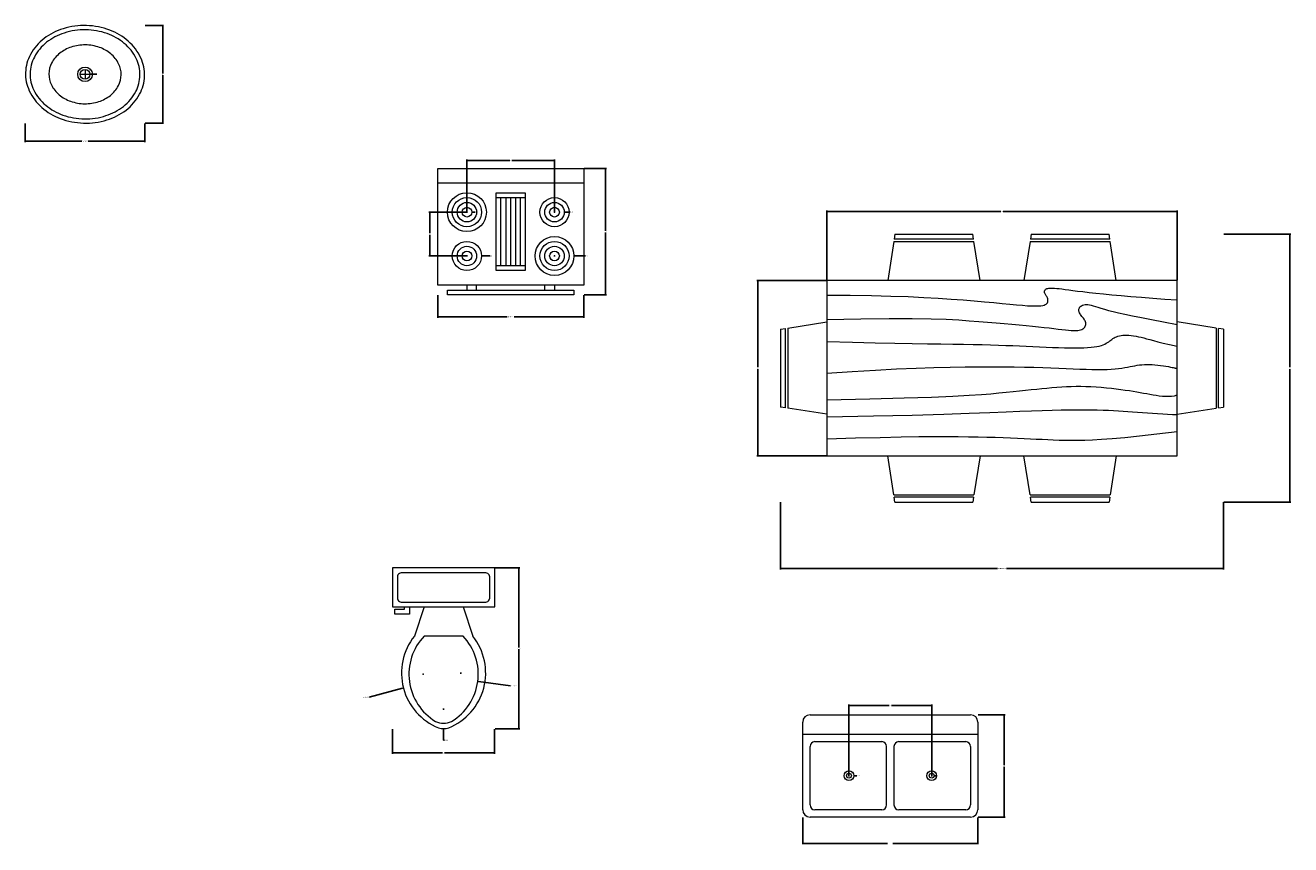
# Model space of a CAD drawing. Units: inches. Extents: x -52 to 1967, y 32 to 824.
# Tile 8 of 10: x 1561 to 1821, y 303 to 471. Entities that reach past the tile are written whole.
import ezdxf

# ---------------------------------------------------------------- set-up
doc = ezdxf.new("R2010")
doc.units = ezdxf.units.IN
for name, color, linetype, lineweight in [('A-ANNO-DIMS', 2, 'Continuous', 18), ('A-EQPM', 9, 'Continuous', 18), ('A-FLOR-FIXT', 9, 'Continuous', 18), ('A-FURN', 8, 'Continuous', 18)]:
    doc.layers.add(name, color=color, linetype=linetype, lineweight=lineweight)
doc.styles.get("Standard").update_dxf_attribs({"font": 'arial.ttf'})
doc.dimstyles.get("Standard").update_dxf_attribs({"dimtxt": 0.18, "dimasz": 0.18, "dimexe": 0.18, "dimexo": 0.0625, "dimgap": 0.09, "dimtad": 0, "dimtih": 1, "dimtoh": 1, "dimdec": 4, "dimzin": 0, "dimdsep": 46, "dimtxsty": 'Standard', "dimcen": 0.09, "dimadec": 0, "dimazin": 0, "dimtfac": 1, "dimtdec": 4, "dimtofl": 0, "dimtmove": 0, "dimatfit": 3, "dimfxl": 1, "dimtolj": 1, "dimtzin": 0, "dimarcsym": 0})

# ---------------------------------------------------------------- blocks, each defined once
blk = doc.blocks.new('Sink-double - 36 in top')
for p, q in [((-18, -4), (18, -4)), ((-0.75, -18.5), (-0.75, -6.5)), ((0.75, -6.5), (0.75, -18.5))]:
    blk.add_line(p, q)
for points in [[(-16.5, 0), (16.5, 0)], [(-18, -19.5), (-18, -1.5)], [(18, -1.5), (18, -19.5)], [(-16.5, -18.5), (-16.5, -6.5)], [(-15.5, -5.5), (-1.75, -5.5)], [(1.75, -5.5), (15.5, -5.5)], [(16.5, -6.5), (16.5, -18.5)], [(-1.75, -19.5), (-15.5, -19.5)], [(15.5, -19.5), (1.75, -19.5)], [(16.5, -21), (-16.5, -21)]]:
    blk.add_lwpolyline(points)
for centre, radius in [((-8.5, -12.5), 1), ((-8.5, -12.5), 0.5), ((8.5, -12.5), 1), ((8.5, -12.5), 0.5)]:
    blk.add_circle(centre, radius)
for centre, radius, start, end in [((-16.5, -1.5), 1.5, 90, 180), ((16.5, -1.5), 1.5, 0, 90), ((-15.5, -6.5), 1, 90, 180), ((-1.75, -6.5), 1, 0, 90), ((1.75, -6.5), 1, 90, 180), ((15.5, -6.5), 1, 0, 90), ((-16.5, -19.5), 1.5, 180, 270), ((-15.5, -18.5), 1, 180, 270), ((-1.75, -18.5), 1, 270, 0), ((1.75, -18.5), 1, 180, 270), ((15.5, -18.5), 1, 270, 0), ((16.5, -19.5), 1.5, 270, 0)]:
    blk.add_arc(centre, radius, start, end)
blk = doc.blocks.new('Range-Oven - 30 in top')
for p, q in [((0, -3), (30, -3)), ((12, -6), (18, -6)), ((13, -20), (13, -6)), ((14, -6), (14, -20)), ((15, -20), (15, -6)), ((16, -6), (16, -20)), ((17, -20), (17, -6)), ((18, -20), (12, -20)), ((6, -24), (6, -25)), ((8, -25), (8, -24)), ((22, -25), (22, -24)), ((24, -24), (24, -25))]:
    blk.add_line(p, q)
for points in [[(0, -24), (0, 0), (30, 0), (30, -24)], [(12, -21), (12, -5), (18, -5), (18, -21)], [(2, -26), (2, -25), (28, -25), (28, -26)]]:
    blk.add_lwpolyline(points, close=True)
for centre, radius in [((6, -9), 4), ((6, -9), 3), ((6, -9), 2), ((24, -9), 3), ((24, -9), 2), ((6, -9), 1), ((24, -9), 1), ((6, -18), 3), ((24, -18), 4), ((24, -18), 3), ((6, -18), 2), ((6, -18), 1), ((24, -18), 2), ((24, -18), 1)]:
    blk.add_circle(centre, radius)
blk = doc.blocks.new('Toilet - top')
for p, q in [((9.5, -6), (9.5, -2)), ((-10, -8.5), (-8, -8.5)), ((-10, -9.5), (-10, -8.5)), ((-7, -9.5), (-10, -9.5)), ((-8, -8.5), (-8, -8)), ((-7, -8), (-7, -9.5)), ((-4, -8), (-6, -14)), ((4, -8), (6, -14)), ((4, -14), (-4, -14))]:
    blk.add_line(p, q)
blk.add_lwpolyline([(10.5, -8), (10.5, 0), (-10.5, 0), (-10.5, -8)], close=True)
for points in [[(-9.5, -2), (-9.5, -6)], [(8.5, -1), (-8.5, -1)], [(-8.5, -7), (8.5, -7)]]:
    blk.add_lwpolyline(points)
for centre, radius, start, end in [((-8.62, -1.88), 0.884, 81.8699, 188.1301), ((8.62, -1.88), 0.884, 351.8699, 98.1301), ((-8.62, -6.12), 0.884, 171.8699, 278.1301), ((8.62, -6.12), 0.884, 261.8699, 8.1301), ((3.52, -21.58), 12.17, 141.4691, 247.9714), ((4.2, -21.82), 11.33, 136.3677, 238.9468), ((-3.52, -21.58), 12.17, 292.0284, 38.5307), ((-4.2, -21.82), 11.33, 301.053, 43.6321), ((0, -27.88), 4, 245.7318, 294.2682), ((0, -29), 4, 254.8605, 285.1395)]:
    blk.add_arc(centre, radius, start, end)
blk = doc.blocks.new('Sink - Oval top')
for p, q in [((-1, 0), (1, 0)), ((0, 1), (0, -1))]:
    blk.add_line(p, q)
for points in [[(-12.23, 0.39, 0.117634), (-11.46, -3.36, 0.104469), (-8.88, -6.8, 0.090016), (-5.08, -9.07, 0.08192), (-0.32, -10.02, 0.08192), (4.49, -9.38, 0.090016), (8.42, -7.36, 0.104469), (11.22, -4.09, 0.117634), (12.23, -0.39, 0.117634), (11.46, 3.36, 0.104469), (8.88, 6.8, 0.090016), (5.08, 9.07, 0.08192), (0.32, 10.02, 0.08192), (-4.49, 9.38, 0.090016), (-8.42, 7.36, 0.104469), (-11.22, 4.09, 0.117634)], [(-11.29, 0.16, 0.118622), (-10.52, -3.25, 0.104678), (-8.07, -6.36, 0.089562), (-4.54, -8.37, 0.081185), (-0.13, -9.15, 0.081185), (4.3, -8.49, 0.089562), (7.89, -6.58, 0.104678), (10.42, -3.55, 0.118622), (11.29, -0.16, 0.118622), (10.52, 3.25, 0.104678), (8.07, 6.36, 0.089562), (4.54, 8.37, 0.081185), (0.13, 9.15, 0.081185), (-4.3, 8.49, 0.089562), (-7.89, 6.58, 0.104678), (-10.42, 3.55, 0.118622)], [(-7.42, 0.08, 0.118283), (-6.91, -2.17, 0.104607), (-5.29, -4.21, 0.089718), (-2.97, -5.53, 0.081436), (-0.07, -6.04, 0.081436), (2.84, -5.59, 0.089718), (5.2, -4.33, 0.104607), (6.86, -2.32, 0.118283), (7.42, -0.08, 0.118283), (6.91, 2.17, 0.104607), (5.29, 4.21, 0.089718), (2.97, 5.53, 0.081436), (0.07, 6.04, 0.081436), (-2.84, 5.59, 0.089718), (-5.2, 4.33, 0.104607), (-6.86, 2.32, 0.118283)]]:
    blk.add_lwpolyline(points, format="xyb", close=True)
for radius in [1.5, 1]:
    blk.add_circle((0, 0), radius)
blk = doc.blocks.new('Dining Set - 36 x 72 in.')
for p, q in [((-22, 27.5), (-22.1562, 26.50042)), ((-5.8416, 26.5), (-22.1534, 26.5)), ((-22, 27.5), (-6, 27.5)), ((-5.8437, 26.49966), (-6, 27.5)), ((6, 27.5), (5.8438, 26.50042)), ((22.1584, 26.5), (5.8466, 26.5)), ((6, 27.5), (22, 27.5)), ((22.1563, 26.49966), (22, 27.5)), ((-22.2343, 26.00059), (-23.4847, 17.99762)), ((-22.2304, 26), (-5.7608, 26)), ((-4.5152, 17.99762), (-5.7655, 25.99926)), ((5.7657, 26.00059), (4.5153, 17.99762)), ((5.7696, 26), (22.2392, 26)), ((23.4848, 17.99762), (22.2345, 25.99926)), ((36, 18), (-36, 18)), ((-36, 18), (-36, -18)), ((36, -18), (36, 18)), ((-45.5, 8), (-44.5004, 8.15617)), ((-45.5, 8), (-45.5, -8)), ((-44.5, -8.15843), (-44.5, 8.15338)), ((-44.0006, 8.23428), (-35.9976, 9.48474)), ((-44, 8.23041), (-44, -8.23915)), ((44.0006, 8.23428), (35.9976, 9.48474)), ((44, 8.23041), (44, -8.23915)), ((44.5, -8.15843), (44.5, 8.15338)), ((45.5, 8), (44.5005, 8.15617)), ((45.5, 8), (45.5, -8)), ((-44.4997, -8.15631), (-45.5, -8)), ((-35.9976, -9.48476), (-43.9993, -8.2345)), ((35.9976, -9.48476), (43.9993, -8.2345)), ((44.4997, -8.15631), (45.5, -8)), ((-36, -18), (36, -18)), ((-22.2343, -26.0006), (-23.4847, -17.99762)), ((-4.5152, -17.99762), (-5.7655, -25.99928)), ((5.7657, -26.0006), (4.5153, -17.99762)), ((23.4848, -17.99762), (22.2345, -25.99928)), ((-22.2304, -26), (-5.7608, -26)), ((5.7696, -26), (22.2392, -26)), ((-22, -27.5), (-22.1562, -26.50044)), ((-5.8416, -26.5), (-22.1534, -26.5)), ((-22, -27.5), (-6, -27.5)), ((-5.8437, -26.49967), (-6, -27.5)), ((6, -27.5), (5.8438, -26.50044)), ((22.1584, -26.5), (5.8466, -26.5)), ((6, -27.5), (22, -27.5)), ((22.1563, -26.49967), (22, -27.5))]:
    blk.add_line(p, q)
for points in [[(-36, 15), (-31.1772, 14.97754), (-26.8079, 14.91406), (-22.8538, 14.81543), (-19.276, 14.6875), (-16.0362, 14.53613), (-13.0957, 14.36718), (-10.4159, 14.18652), (-7.9583, 14), (-5.6904, 13.81315), (-3.6035, 13.63021), (-1.6954, 13.45508), (0.0365, 13.29166), (1.5945, 13.14388), (2.9811, 13.01562), (4.1988, 12.9108), (5.25, 12.83333), (6.1393, 12.78613), (6.8802, 12.76823), (7.4883, 12.77767), (7.9792, 12.8125), (8.3685, 12.87077), (8.6719, 12.95052), (8.9049, 13.0498), (9.0833, 13.16666), (9.2205, 13.29899), (9.3216, 13.44401), (9.3895, 13.59879), (9.4271, 13.76041), (9.4373, 13.92594), (9.4232, 14.09245), (9.3875, 14.257), (9.3333, 14.41666), (9.2638, 14.56917), (9.1836, 14.71484), (9.0975, 14.85465), (9.0104, 14.98958), (8.9272, 15.1206), (8.8529, 15.2487), (8.7922, 15.37483), (8.75, 15.5), (8.7305, 15.62467), (8.7344, 15.74739), (8.7617, 15.86621), (8.8125, 15.97916), (8.8867, 16.08431), (8.9844, 16.17968), (9.1055, 16.26334), (9.25, 16.33333), (9.4189, 16.38802), (9.6172, 16.42708), (9.8506, 16.45052), (10.125, 16.45833), (10.4463, 16.45052), (10.8203, 16.42708), (11.2529, 16.38802), (11.75, 16.33333), (12.3184, 16.26318), (12.9694, 16.17838), (13.7151, 16.07991), (14.5677, 15.96875), (15.5395, 15.84586), (16.6426, 15.71224), (17.8893, 15.56884), (19.2917, 15.41666), (20.859, 15.25667), (22.5879, 15.08984), (24.4721, 14.91715), (26.5052, 14.73958), (28.6809, 14.5581), (30.9929, 14.3737), (33.4347, 14.18733), (36, 14)], [(-36, 10), (-28.9766, 10.14274), (-23.1725, 10.20442), (-18.4241, 10.19775), (-14.5677, 10.13541), (-11.4399, 10.03011), (-8.877, 9.89453), (-6.7154, 9.74137), (-4.7917, 9.58333), (-2.9698, 9.43082), (-1.2246, 9.28515), (0.4415, 9.14534), (2.026, 9.01041), (3.5266, 8.87939), (4.9408, 8.7513), (6.266, 8.62516), (7.5, 8.5), (8.6411, 8.37549), (9.6914, 8.2539), (10.6538, 8.13818), (11.5312, 8.03125), (12.3267, 7.93603), (13.043, 7.85547), (13.6831, 7.79248), (14.25, 7.75), (14.7471, 7.7303), (15.1797, 7.73307), (15.5537, 7.75732), (15.875, 7.80208), (16.1494, 7.86637), (16.3828, 7.94922), (16.5811, 8.04964), (16.75, 8.16666), (16.8944, 8.29915), (17.0143, 8.44531), (17.1089, 8.60319), (17.1771, 8.77083), (17.218, 8.94629), (17.2305, 9.1276), (17.2137, 9.31282), (17.1667, 9.5), (17.0895, 9.6875), (16.987, 9.875), (16.8649, 10.0625), (16.7292, 10.25), (16.5856, 10.4375), (16.4401, 10.625), (16.2985, 10.8125), (16.1667, 11), (16.05, 11.18733), (15.9518, 11.3737), (15.8752, 11.5581), (15.8229, 11.73958), (15.798, 11.91715), (15.8034, 12.08984), (15.842, 12.25667), (15.9167, 12.41666), (16.0295, 12.56836), (16.1784, 12.70833), (16.3605, 12.83268), (16.5729, 12.9375), (16.8127, 13.01888), (17.0768, 13.07291), (17.3625, 13.0957), (17.6667, 13.08333), (17.9894, 13.03312), (18.3418, 12.94726), (18.7382, 12.82918), (19.1927, 12.68229), (19.7195, 12.51001), (20.3327, 12.31575), (21.0465, 12.10294), (21.875, 11.875), (22.8357, 11.63354), (23.959, 11.37304), (25.2786, 11.08618), (26.8282, 10.76562), (28.6414, 10.40405), (30.752, 9.99414), (33.1936, 9.52856), (36, 9)], [(-36, 5.5), (-30.7157, 5.3348), (-26.069, 5.20963), (-21.9946, 5.11767), (-18.4271, 5.05208), (-15.3009, 5.00602), (-12.5508, 4.97265), (-10.1112, 4.94515), (-7.9167, 4.91666), (-5.909, 4.88167), (-4.0586, 4.83984), (-2.3429, 4.79215), (-0.7396, 4.73958), (0.7739, 4.6831), (2.22, 4.6237), (3.6213, 4.56233), (5, 4.5), (6.373, 4.43782), (7.7344, 4.3776), (9.0723, 4.32129), (10.375, 4.27083), (11.6309, 4.22819), (12.8281, 4.19531), (13.9551, 4.17415), (15, 4.16666), (15.954, 4.17448), (16.819, 4.19791), (17.6001, 4.23698), (18.3021, 4.29166), (18.9299, 4.36198), (19.4883, 4.44791), (19.9823, 4.54948), (20.4167, 4.66666), (20.7969, 4.79899), (21.1302, 4.94401), (21.4245, 5.09879), (21.6875, 5.26041), (21.9271, 5.42594), (22.1511, 5.59245), (22.3672, 5.757), (22.5834, 5.91666), (22.8065, 6.06868), (23.0404, 6.21093), (23.2879, 6.34147), (23.5521, 6.45833), (23.8358, 6.55957), (24.142, 6.64323), (24.4735, 6.70735), (24.8334, 6.75), (25.2235, 6.76969), (25.642, 6.76692), (26.0858, 6.74267), (26.5521, 6.69791), (27.0379, 6.63362), (27.5404, 6.55078), (28.0565, 6.45036), (28.5834, 6.33333), (29.1242, 6.19987), (29.7071, 6.04687), (30.3661, 5.87044), (31.1354, 5.66666), (32.0493, 5.43164), (33.142, 5.16146), (34.4475, 4.85221), (36, 4.5)], [(-36, -1), (-30.7915, -0.6591), (-26.0195, -0.38216), (-21.6519, -0.16284), (-17.6563, 0.00521), (-14.0005, 0.12833), (-10.6523, 0.21289), (-7.5796, 0.26522), (-4.75, 0.29166), (-2.134, 0.29793), (0.2878, 0.28711), (2.5317, 0.26163), (4.6146, 0.22396), (6.5529, 0.17651), (8.3633, 0.12174), (10.0623, 0.06209), (11.6667, 0), (13.1899, -0.06201), (14.6341, -0.1211), (15.9982, -0.17432), (17.2813, -0.21875), (18.4823, -0.25147), (19.6003, -0.26953), (20.6343, -0.27002), (21.5834, -0.25), (22.4481, -0.20768), (23.2357, -0.14584), (23.9549, -0.06836), (24.6146, 0.02083), (25.2235, 0.11784), (25.7904, 0.21875), (26.3241, 0.31966), (26.8334, 0.41666), (27.3265, 0.50618), (27.8099, 0.58593), (28.2894, 0.65397), (28.7709, 0.70833), (29.2601, 0.74707), (29.763, 0.76823), (30.2855, 0.76985), (30.8334, 0.75), (31.4088, 0.70784), (31.9994, 0.64713), (32.589, 0.57275), (33.1615, 0.48958), (33.7008, 0.4025), (34.1908, 0.3164), (34.6153, 0.23616), (34.9584, 0.16666), (35.2099, 0.11165), (35.3848, 0.07031), (35.504, 0.04069), (35.5886, 0.02083), (35.6594, 0.00879), (35.7377, 0.0026), (35.8442, 0.00032), (36, 0)], [(-36, -6.5), (-27.1843, -6.31267), (-20.084, -6.1263), (-14.469, -5.9419), (-10.1094, -5.76042), (-6.7752, -5.58285), (-4.2363, -5.41016), (-2.2629, -5.24333), (-0.625, -5.08334), (0.8708, -4.93099), (2.2715, -4.78646), (3.5872, -4.64974), (4.8281, -4.52084), (6.0046, -4.39974), (7.127, -4.28646), (8.2053, -4.18099), (9.25, -4.08334), (10.2705, -3.99382), (11.2734, -3.91407), (12.2647, -3.84603), (13.25, -3.79167), (14.2354, -3.75293), (15.2266, -3.73177), (16.2295, -3.73015), (17.25, -3.75), (18.2912, -3.79248), (19.3451, -3.85547), (20.4009, -3.93604), (21.4479, -4.03125), (22.4754, -4.13819), (23.4727, -4.25391), (24.4289, -4.37549), (25.3334, -4.5), (26.1785, -4.62492), (26.9694, -4.74935), (27.7145, -4.87281), (28.4219, -4.99479), (29.1, -5.11483), (29.7572, -5.23242), (30.4016, -5.34709), (31.0417, -5.45834), (31.6837, -5.56437), (32.3262, -5.65821), (32.9658, -5.73153), (33.599, -5.77604), (34.2224, -5.78345), (34.8327, -5.74545), (35.4264, -5.65373), (36, -5.5)], [(-36, -10), (-26.4022, -9.81299), (-18.4675, -9.62891), (-11.9839, -9.45069), (-6.7396, -9.28125), (-2.5226, -9.12354), (0.8789, -8.98047), (3.6769, -8.85498), (6.0833, -8.75), (8.2767, -8.66765), (10.3021, -8.60677), (12.1712, -8.56543), (13.8958, -8.54167), (15.4876, -8.53353), (16.9583, -8.53907), (18.3197, -8.55632), (19.5834, -8.58334), (20.7616, -8.61841), (21.8685, -8.66081), (22.9188, -8.71004), (23.9271, -8.76563), (24.9081, -8.82707), (25.8763, -8.89388), (26.8465, -8.96558), (27.8334, -9.04167), (28.8474, -9.12118), (29.8828, -9.20117), (30.93, -9.27824), (31.9792, -9.34896), (33.0205, -9.40991), (34.0443, -9.45768), (35.0407, -9.48885), (36, -9.5)], [(-36, -14.5), (-30.0881, -14.33513), (-25.0332, -14.21224), (-20.7312, -14.12647), (-17.0781, -14.07292), (-13.97, -14.04671), (-11.3027, -14.04297), (-8.9724, -14.05681), (-6.875, -14.08334), (-4.9224, -14.11833), (-3.0905, -14.16016), (-1.3709, -14.20785), (0.2448, -14.26042), (1.7647, -14.3169), (3.1973, -14.3763), (4.5507, -14.43767), (5.8333, -14.5), (7.0554, -14.5621), (8.235, -14.62175), (9.3922, -14.67652), (10.5469, -14.72396), (11.7192, -14.76164), (12.929, -14.78711), (14.1965, -14.79794), (15.5417, -14.79167), (16.9933, -14.76424), (18.6152, -14.70508), (20.4804, -14.60197), (22.6615, -14.44271), (25.2312, -14.21509), (28.2624, -13.9069), (31.8277, -13.50594), (36, -13)]]:
    blk.add_lwpolyline(points)
blk = doc.blocks.new('*D37')
at = {"layer": 'A-ANNO-DIMS', "color": 0, "lineweight": -2, "transparency": 16777216}
for p, q in [((1715.93, 373.48), (1715.93, 359.71)), ((1806.93, 373.48), (1806.93, 359.71)), ((1716.11, 359.89), (1760.47, 359.89)), ((1806.75, 359.89), (1762.38, 359.89))]:
    blk.add_line(p, q, dxfattribs=at)
at = {"layer": 'A-ANNO-DIMS', "color": 0, "transparency": 16777216}
for points in [[(1716.11, 359.92), (1716.11, 359.86), (1715.93, 359.89)], [(1806.75, 359.92), (1806.75, 359.86), (1806.93, 359.89)]]:
    blk.add_solid(points, dxfattribs=at)
at = {"layer": 'Defpoints', "color": 0, "transparency": 16777216}
for p in [(1715.93, 373.54), (1806.93, 373.54), (1806.93, 359.89)]:
    blk.add_point(p, dxfattribs=at)
at = {"layer": 'A-ANNO-DIMS', "color": 0, "transparency": 16777216, "insert": (1761.43, 359.89), "char_height": 0.18, "attachment_point": 5}
blk.add_mtext('\\A1;DINING SET 91', dxfattribs=at)
blk = doc.blocks.new('*D38')
at = {"layer": 'A-ANNO-DIMS', "color": 0, "lineweight": -2, "transparency": 16777216}
for p, q in [((1806.99, 428.54), (1820.76, 428.54)), ((1820.58, 428.36), (1820.58, 401.22)), ((1820.58, 373.72), (1820.58, 400.86)), ((1806.99, 373.54), (1820.76, 373.54))]:
    blk.add_line(p, q, dxfattribs=at)
at = {"layer": 'A-ANNO-DIMS', "color": 0, "transparency": 16777216}
for points in [[(1820.55, 428.36), (1820.61, 428.36), (1820.58, 428.54)], [(1820.55, 373.72), (1820.61, 373.72), (1820.58, 373.54)]]:
    blk.add_solid(points, dxfattribs=at)
at = {"layer": 'Defpoints', "color": 0, "transparency": 16777216}
for p in [(1806.93, 428.54), (1820.58, 428.54), (1806.93, 373.54)]:
    blk.add_point(p, dxfattribs=at)
at = {"layer": 'A-ANNO-DIMS', "color": 0, "transparency": 16777216, "insert": (1820.58, 401.04), "char_height": 0.18, "attachment_point": 5}
blk.add_mtext('\\A1;55', dxfattribs=at)
blk = doc.blocks.new('*D41')
at = {"layer": 'A-ANNO-DIMS', "color": 0, "lineweight": -2, "transparency": 16777216}
for p, q in [((1657.24, 360), (1662.31, 360)), ((1662.13, 359.82), (1662.13, 343.66)), ((1662.13, 327.13), (1662.13, 343.29)), ((1657.24, 326.95), (1662.31, 326.95))]:
    blk.add_line(p, q, dxfattribs=at)
at = {"layer": 'A-ANNO-DIMS', "color": 0, "transparency": 16777216}
for points in [[(1662.1, 359.82), (1662.16, 359.82), (1662.13, 360)], [(1662.1, 327.13), (1662.16, 327.13), (1662.13, 326.95)]]:
    blk.add_solid(points, dxfattribs=at)
at = {"layer": 'Defpoints', "color": 0, "transparency": 16777216}
for p in [(1657.17, 360), (1662.13, 360), (1657.17, 326.95)]:
    blk.add_point(p, dxfattribs=at)
at = {"layer": 'A-ANNO-DIMS', "color": 0, "transparency": 16777216, "insert": (1662.13, 343.47), "char_height": 0.18, "attachment_point": 5}
blk.add_mtext('\\A1;WC 33', dxfattribs=at)
blk = doc.blocks.new('*D42')
at = {"layer": 'A-ANNO-DIMS', "color": 0, "lineweight": -2, "transparency": 16777216}
for p, q in [((1636.17, 326.89), (1636.17, 321.81)), ((1657.17, 326.89), (1657.17, 321.81)), ((1636.35, 321.99), (1646.47, 321.99)), ((1656.99, 321.99), (1646.88, 321.99))]:
    blk.add_line(p, q, dxfattribs=at)
at = {"layer": 'A-ANNO-DIMS', "color": 0, "transparency": 16777216}
for points in [[(1636.35, 322.02), (1636.35, 321.96), (1636.17, 321.99)], [(1656.99, 322.02), (1656.99, 321.96), (1657.17, 321.99)]]:
    blk.add_solid(points, dxfattribs=at)
at = {"layer": 'Defpoints', "color": 0, "transparency": 16777216}
for p in [(1636.17, 326.95), (1657.17, 326.95), (1657.17, 321.99)]:
    blk.add_point(p, dxfattribs=at)
at = {"layer": 'A-ANNO-DIMS', "color": 0, "transparency": 16777216, "insert": (1646.67, 321.99), "char_height": 0.18, "attachment_point": 5}
blk.add_mtext('\\A1;21', dxfattribs=at)
blk = doc.blocks.new('*D43')
at = {"layer": 'A-ANNO-DIMS', "color": 0, "lineweight": -2, "transparency": 16777216}
for p, q in [((1560.72, 451.27), (1560.72, 447.47)), ((1585.27, 451.27), (1585.27, 447.47)), ((1560.9, 447.65), (1572.36, 447.65)), ((1585.09, 447.65), (1573.62, 447.65))]:
    blk.add_line(p, q, dxfattribs=at)
at = {"layer": 'A-ANNO-DIMS', "color": 0, "transparency": 16777216}
for points in [[(1560.9, 447.68), (1560.9, 447.62), (1560.72, 447.65)], [(1585.09, 447.68), (1585.09, 447.62), (1585.27, 447.65)]]:
    blk.add_solid(points, dxfattribs=at)
at = {"layer": 'Defpoints', "color": 0, "transparency": 16777216}
for p in [(1560.72, 451.33), (1585.27, 451.33), (1585.27, 447.65)]:
    blk.add_point(p, dxfattribs=at)
at = {"layer": 'A-ANNO-DIMS', "color": 0, "transparency": 16777216, "insert": (1572.99, 447.65), "char_height": 0.18, "attachment_point": 5}
blk.add_mtext('\\A1;BASIN 25', dxfattribs=at)
blk = doc.blocks.new('*D44')
at = {"layer": 'A-ANNO-DIMS', "color": 0, "lineweight": -2, "transparency": 16777216}
for p, q in [((1585.33, 471.46), (1589.13, 471.46)), ((1588.95, 471.28), (1588.95, 461.58)), ((1588.95, 451.51), (1588.95, 461.21)), ((1585.33, 451.33), (1589.13, 451.33))]:
    blk.add_line(p, q, dxfattribs=at)
at = {"layer": 'A-ANNO-DIMS', "color": 0, "transparency": 16777216}
for points in [[(1588.92, 471.28), (1588.98, 471.28), (1588.95, 471.46)], [(1588.92, 451.51), (1588.98, 451.51), (1588.95, 451.33)]]:
    blk.add_solid(points, dxfattribs=at)
at = {"layer": 'Defpoints', "color": 0, "transparency": 16777216}
for p in [(1585.27, 471.46), (1588.95, 471.46), (1585.27, 451.33)]:
    blk.add_point(p, dxfattribs=at)
at = {"layer": 'A-ANNO-DIMS', "color": 0, "transparency": 16777216, "insert": (1588.95, 461.4), "char_height": 0.18, "attachment_point": 5}
blk.add_mtext('\\A1;20', dxfattribs=at)
blk = doc.blocks.new('*D45')
at = {"layer": 'A-ANNO-DIMS', "color": 0, "lineweight": -2, "transparency": 16777216}
for p, q in [((1720.48, 308.75), (1720.48, 303.24)), ((1756.48, 308.75), (1756.48, 303.24)), ((1720.66, 303.42), (1737.93, 303.42)), ((1756.3, 303.42), (1739.02, 303.42))]:
    blk.add_line(p, q, dxfattribs=at)
at = {"layer": 'A-ANNO-DIMS', "color": 0, "transparency": 16777216}
for points in [[(1720.66, 303.45), (1720.66, 303.39), (1720.48, 303.42)], [(1756.3, 303.45), (1756.3, 303.39), (1756.48, 303.42)]]:
    blk.add_solid(points, dxfattribs=at)
at = {"layer": 'Defpoints', "color": 0, "transparency": 16777216}
for p in [(1720.48, 308.82), (1756.48, 308.82), (1756.48, 303.42)]:
    blk.add_point(p, dxfattribs=at)
at = {"layer": 'A-ANNO-DIMS', "color": 0, "transparency": 16777216, "insert": (1738.48, 303.42), "char_height": 0.18, "attachment_point": 5}
blk.add_mtext('\\A1;SINK 36', dxfattribs=at)
blk = doc.blocks.new('*D46')
at = {"layer": 'A-ANNO-DIMS', "color": 0, "lineweight": -2, "transparency": 16777216}
for p, q in [((1756.54, 329.82), (1762.06, 329.82)), ((1761.88, 329.64), (1761.88, 319.5)), ((1761.88, 309), (1761.88, 319.14)), ((1756.54, 308.82), (1762.06, 308.82))]:
    blk.add_line(p, q, dxfattribs=at)
at = {"layer": 'A-ANNO-DIMS', "color": 0, "transparency": 16777216}
for points in [[(1761.85, 329.64), (1761.91, 329.64), (1761.88, 329.82)], [(1761.85, 309), (1761.91, 309), (1761.88, 308.82)]]:
    blk.add_solid(points, dxfattribs=at)
at = {"layer": 'Defpoints', "color": 0, "transparency": 16777216}
for p in [(1756.48, 329.82), (1761.88, 329.82), (1756.48, 308.82)]:
    blk.add_point(p, dxfattribs=at)
at = {"layer": 'A-ANNO-DIMS', "color": 0, "transparency": 16777216, "insert": (1761.88, 319.32), "char_height": 0.18, "attachment_point": 5}
blk.add_mtext('\\A1;21', dxfattribs=at)
blk = doc.blocks.new('*D47')
at = {"layer": 'A-ANNO-DIMS', "color": 0, "lineweight": -2, "transparency": 16777216}
for p, q in [((1645.47, 416.02), (1645.47, 411.4)), ((1675.47, 416.02), (1675.47, 411.4)), ((1645.65, 411.58), (1659.77, 411.58)), ((1675.29, 411.58), (1661.16, 411.58))]:
    blk.add_line(p, q, dxfattribs=at)
at = {"layer": 'A-ANNO-DIMS', "color": 0, "transparency": 16777216}
for points in [[(1645.65, 411.61), (1645.65, 411.55), (1645.47, 411.58)], [(1675.29, 411.61), (1675.29, 411.55), (1675.47, 411.58)]]:
    blk.add_solid(points, dxfattribs=at)
at = {"layer": 'Defpoints', "color": 0, "transparency": 16777216}
for p in [(1645.47, 416.08), (1675.47, 416.08), (1675.47, 411.58)]:
    blk.add_point(p, dxfattribs=at)
at = {"layer": 'A-ANNO-DIMS', "color": 0, "transparency": 16777216, "insert": (1660.47, 411.58), "char_height": 0.18, "attachment_point": 5}
blk.add_mtext('\\A1;RANGE 30', dxfattribs=at)
blk = doc.blocks.new('*D48')
at = {"layer": 'A-ANNO-DIMS', "color": 0, "lineweight": -2, "transparency": 16777216}
for p, q in [((1675.53, 442.08), (1680.15, 442.08)), ((1679.97, 441.9), (1679.97, 429.26)), ((1679.97, 416.26), (1679.97, 428.9)), ((1675.53, 416.08), (1680.15, 416.08))]:
    blk.add_line(p, q, dxfattribs=at)
at = {"layer": 'A-ANNO-DIMS', "color": 0, "transparency": 16777216}
for points in [[(1679.94, 441.9), (1680, 441.9), (1679.97, 442.08)], [(1679.94, 416.26), (1680, 416.26), (1679.97, 416.08)]]:
    blk.add_solid(points, dxfattribs=at)
at = {"layer": 'Defpoints', "color": 0, "transparency": 16777216}
for p in [(1675.47, 442.08), (1679.97, 442.08), (1675.47, 416.08)]:
    blk.add_point(p, dxfattribs=at)
at = {"layer": 'A-ANNO-DIMS', "color": 0, "transparency": 16777216, "insert": (1679.97, 429.08), "char_height": 0.18, "attachment_point": 5}
blk.add_mtext('\\A1;26', dxfattribs=at)
blk = doc.blocks.new('*D126')
at = {"layer": 'A-ANNO-DIMS', "color": 0, "lineweight": -2, "transparency": 16777216}
for p, q in [((1725.43, 419.1), (1725.43, 433.41)), ((1725.61, 433.23), (1761.21, 433.23)), ((1797.25, 433.23), (1761.64, 433.23)), ((1797.43, 419.1), (1797.43, 433.41))]:
    blk.add_line(p, q, dxfattribs=at)
at = {"layer": 'A-ANNO-DIMS', "color": 0, "transparency": 16777216}
for points in [[(1725.61, 433.26), (1725.61, 433.2), (1725.43, 433.23)], [(1797.25, 433.26), (1797.25, 433.2), (1797.43, 433.23)]]:
    blk.add_solid(points, dxfattribs=at)
at = {"layer": 'Defpoints', "color": 0, "transparency": 16777216}
for p in [(1797.43, 433.23), (1725.43, 419.04), (1797.43, 419.04)]:
    blk.add_point(p, dxfattribs=at)
at = {"layer": 'A-ANNO-DIMS', "color": 0, "transparency": 16777216, "insert": (1761.43, 433.23), "char_height": 0.18, "attachment_point": 5}
blk.add_mtext('\\A1;72', dxfattribs=at)
blk = doc.blocks.new('*D127')
at = {"layer": 'A-ANNO-DIMS', "color": 0, "lineweight": -2, "transparency": 16777216}
for p, q in [((1725.36, 419.04), (1711.06, 419.04)), ((1711.24, 418.86), (1711.24, 401.22)), ((1711.24, 383.22), (1711.24, 400.86)), ((1725.36, 383.04), (1711.06, 383.04))]:
    blk.add_line(p, q, dxfattribs=at)
at = {"layer": 'A-ANNO-DIMS', "color": 0, "transparency": 16777216}
for points in [[(1711.21, 418.86), (1711.27, 418.86), (1711.24, 419.04)], [(1711.21, 383.22), (1711.27, 383.22), (1711.24, 383.04)]]:
    blk.add_solid(points, dxfattribs=at)
at = {"layer": 'Defpoints', "color": 0, "transparency": 16777216}
for p in [(1711.24, 419.04), (1725.43, 419.04), (1725.43, 383.04)]:
    blk.add_point(p, dxfattribs=at)
at = {"layer": 'A-ANNO-DIMS', "color": 0, "transparency": 16777216, "insert": (1711.24, 401.04), "char_height": 0.18, "attachment_point": 5}
blk.add_mtext('\\A1;36', dxfattribs=at)
blk = doc.blocks.new('*D128')
at = {"layer": 'A-ANNO-DIMS', "color": 0, "lineweight": -2, "transparency": 16777216}
for p, q in [((1651.47, 433.14), (1651.47, 443.9)), ((1651.65, 443.72), (1660.26, 443.72)), ((1669.29, 443.72), (1660.68, 443.72)), ((1669.47, 433.14), (1669.47, 443.9))]:
    blk.add_line(p, q, dxfattribs=at)
at = {"layer": 'A-ANNO-DIMS', "color": 0, "transparency": 16777216}
for points in [[(1651.65, 443.75), (1651.65, 443.69), (1651.47, 443.72)], [(1669.29, 443.75), (1669.29, 443.69), (1669.47, 443.72)]]:
    blk.add_solid(points, dxfattribs=at)
at = {"layer": 'Defpoints', "color": 0, "transparency": 16777216}
for p in [(1669.47, 443.72), (1651.47, 433.08), (1669.47, 433.08)]:
    blk.add_point(p, dxfattribs=at)
at = {"layer": 'A-ANNO-DIMS', "color": 0, "transparency": 16777216, "insert": (1660.47, 443.72), "char_height": 0.18, "attachment_point": 5}
blk.add_mtext('\\A1;18', dxfattribs=at)
blk = doc.blocks.new('*D129')
at = {"layer": 'A-ANNO-DIMS', "color": 0, "lineweight": -2, "transparency": 16777216}
for p, q in [((1651.4, 433.08), (1643.65, 433.08)), ((1643.83, 432.9), (1643.83, 428.76)), ((1643.83, 424.26), (1643.83, 428.4)), ((1651.4, 424.08), (1643.65, 424.08))]:
    blk.add_line(p, q, dxfattribs=at)
at = {"layer": 'A-ANNO-DIMS', "color": 0, "transparency": 16777216}
for points in [[(1643.8, 432.9), (1643.86, 432.9), (1643.83, 433.08)], [(1643.8, 424.26), (1643.86, 424.26), (1643.83, 424.08)]]:
    blk.add_solid(points, dxfattribs=at)
at = {"layer": 'Defpoints', "color": 0, "transparency": 16777216}
for p in [(1643.83, 433.08), (1651.47, 433.08), (1651.47, 424.08)]:
    blk.add_point(p, dxfattribs=at)
at = {"layer": 'A-ANNO-DIMS', "color": 0, "transparency": 16777216, "insert": (1643.83, 428.58), "char_height": 0.18, "attachment_point": 5}
blk.add_mtext('\\A1;9', dxfattribs=at)
blk = doc.blocks.new('*D132')
at = {"layer": 'A-ANNO-DIMS', "color": 0, "lineweight": -2, "transparency": 16777216}
for p, q in [((1729.98, 317.38), (1729.98, 331.95)), ((1730.16, 331.77), (1738.27, 331.77)), ((1746.8, 331.77), (1738.69, 331.77)), ((1746.98, 317.38), (1746.98, 331.95))]:
    blk.add_line(p, q, dxfattribs=at)
at = {"layer": 'A-ANNO-DIMS', "color": 0, "transparency": 16777216}
for points in [[(1730.16, 331.8), (1730.16, 331.74), (1729.98, 331.77)], [(1746.8, 331.8), (1746.8, 331.74), (1746.98, 331.77)]]:
    blk.add_solid(points, dxfattribs=at)
at = {"layer": 'Defpoints', "color": 0, "transparency": 16777216}
for p in [(1746.98, 331.77), (1729.98, 317.32), (1746.98, 317.32)]:
    blk.add_point(p, dxfattribs=at)
at = {"layer": 'A-ANNO-DIMS', "color": 0, "transparency": 16777216, "insert": (1738.48, 331.77), "char_height": 0.18, "attachment_point": 5}
blk.add_mtext('\\A1;17', dxfattribs=at)
blk = doc.blocks.new('*D152')
at = {"layer": 'A-ANNO-DIMS', "color": 0, "lineweight": -2, "transparency": 16777216}
for p, q in [((1650.1, 338.41), (1650.28, 338.41)), ((1650.19, 338.32), (1650.19, 338.5)), ((1631.36, 333.47), (1638.25, 335.28))]:
    blk.add_line(p, q, dxfattribs=at)
at = {"layer": 'A-ANNO-DIMS', "color": 0, "transparency": 16777216}
blk.add_solid([(1638.24, 335.31), (1638.26, 335.25), (1638.42, 335.32)], dxfattribs=at)
at = {"layer": 'Defpoints', "color": 0, "transparency": 16777216}
for p in [(1650.19, 338.41), (1638.42, 335.32)]:
    blk.add_point(p, dxfattribs=at)
at = {"layer": 'A-ANNO-DIMS', "color": 0, "transparency": 16777216, "insert": (1630.69, 333.47), "char_height": 0.18, "attachment_point": 5}
blk.add_mtext('\\A1;2X R12.17', dxfattribs=at)
blk = doc.blocks.new('*D153')
at = {"layer": 'A-ANNO-DIMS', "color": 0, "lineweight": -2, "transparency": 16777216}
for p, q in [((1642.38, 338.18), (1642.56, 338.18)), ((1642.47, 338.09), (1642.47, 338.27)), ((1660.44, 335.76), (1653.88, 336.64))]:
    blk.add_line(p, q, dxfattribs=at)
at = {"layer": 'A-ANNO-DIMS', "color": 0, "transparency": 16777216}
blk.add_solid([(1653.88, 336.67), (1653.88, 336.61), (1653.7, 336.67)], dxfattribs=at)
at = {"layer": 'Defpoints', "color": 0, "transparency": 16777216}
for p in [(1642.47, 338.18), (1653.7, 336.67)]:
    blk.add_point(p, dxfattribs=at)
at = {"layer": 'A-ANNO-DIMS', "color": 0, "transparency": 16777216, "insert": (1661.11, 335.76), "char_height": 0.18, "attachment_point": 5}
blk.add_mtext('\\A1;2X R11.33', dxfattribs=at)
blk = doc.blocks.new('*D154')
at = {"layer": 'A-ANNO-DIMS', "color": 0, "lineweight": -2, "transparency": 16777216}
for p, q in [((1646.58, 331), (1646.76, 331)), ((1646.67, 330.91), (1646.67, 331.09)), ((1646.67, 324.6), (1646.67, 326.82)), ((1646.85, 324.6), (1646.67, 324.6))]:
    blk.add_line(p, q, dxfattribs=at)
at = {"layer": 'A-ANNO-DIMS', "color": 0, "transparency": 16777216}
blk.add_solid([(1646.7, 326.82), (1646.64, 326.82), (1646.67, 327)], dxfattribs=at)
at = {"layer": 'Defpoints', "color": 0, "transparency": 16777216}
for p in [(1646.67, 331), (1646.67, 327)]:
    blk.add_point(p, dxfattribs=at)
at = {"layer": 'A-ANNO-DIMS', "color": 0, "transparency": 16777216, "insert": (1647.28, 324.6), "char_height": 0.18, "attachment_point": 5}
blk.add_mtext('\\A1;2X R4', dxfattribs=at)
blk = doc.blocks.new('*D155')
at = {"layer": 'A-ANNO-DIMS', "color": 0, "lineweight": -2, "transparency": 16777216}
for p, q in [((1669.38, 424.08), (1669.56, 424.08)), ((1669.47, 423.99), (1669.47, 424.17)), ((1675.87, 424.08), (1673.65, 424.08))]:
    blk.add_line(p, q, dxfattribs=at)
at = {"layer": 'A-ANNO-DIMS', "color": 0, "transparency": 16777216}
blk.add_solid([(1673.65, 424.11), (1673.65, 424.05), (1673.47, 424.08)], dxfattribs=at)
at = {"layer": 'Defpoints', "color": 0, "transparency": 16777216}
for p in [(1665.47, 424.08), (1673.47, 424.08)]:
    blk.add_point(p, dxfattribs=at)
at = {"layer": 'A-ANNO-DIMS', "color": 0, "transparency": 16777216, "insert": (1676.3, 424.08), "char_height": 0.18, "attachment_point": 5}
blk.add_mtext('\\A1;2X ∅8', dxfattribs=at)
blk = doc.blocks.new('*D156')
at = {"layer": 'A-ANNO-DIMS', "color": 0, "lineweight": -2, "transparency": 16777216}
for p, q in [((1651.38, 424.08), (1651.56, 424.08)), ((1651.47, 423.99), (1651.47, 424.17)), ((1656.27, 424.08), (1654.65, 424.08))]:
    blk.add_line(p, q, dxfattribs=at)
at = {"layer": 'A-ANNO-DIMS', "color": 0, "transparency": 16777216}
blk.add_solid([(1654.65, 424.11), (1654.65, 424.05), (1654.47, 424.08)], dxfattribs=at)
at = {"layer": 'Defpoints', "color": 0, "transparency": 16777216}
for p in [(1648.47, 424.08), (1654.47, 424.08)]:
    blk.add_point(p, dxfattribs=at)
at = {"layer": 'A-ANNO-DIMS', "color": 0, "transparency": 16777216, "insert": (1656.71, 424.08), "char_height": 0.18, "attachment_point": 5}
blk.add_mtext('\\A1;4X ∅6', dxfattribs=at)
blk = doc.blocks.new('*D157')
at = {"layer": 'A-ANNO-DIMS', "color": 0, "lineweight": -2, "transparency": 16777216}
for p, q in [((1669.38, 433.08), (1669.56, 433.08)), ((1669.47, 432.99), (1669.47, 433.17)), ((1672.67, 433.08), (1671.65, 433.08))]:
    blk.add_line(p, q, dxfattribs=at)
at = {"layer": 'A-ANNO-DIMS', "color": 0, "transparency": 16777216}
blk.add_solid([(1671.65, 433.11), (1671.65, 433.05), (1671.47, 433.08)], dxfattribs=at)
at = {"layer": 'Defpoints', "color": 0, "transparency": 16777216}
for p in [(1667.47, 433.08), (1671.47, 433.08)]:
    blk.add_point(p, dxfattribs=at)
at = {"layer": 'A-ANNO-DIMS', "color": 0, "transparency": 16777216, "insert": (1673.1, 433.08), "char_height": 0.18, "attachment_point": 5}
blk.add_mtext('\\A1;4X ∅4', dxfattribs=at)
blk = doc.blocks.new('*D158')
at = {"layer": 'A-ANNO-DIMS', "color": 0, "lineweight": -2, "transparency": 16777216}
for p, q in [((1651.38, 433.08), (1651.56, 433.08)), ((1651.47, 432.99), (1651.47, 433.17)), ((1653.07, 433.08), (1652.65, 433.08))]:
    blk.add_line(p, q, dxfattribs=at)
at = {"layer": 'A-ANNO-DIMS', "color": 0, "transparency": 16777216}
blk.add_solid([(1652.65, 433.11), (1652.65, 433.05), (1652.47, 433.08)], dxfattribs=at)
at = {"layer": 'Defpoints', "color": 0, "transparency": 16777216}
for p in [(1650.47, 433.08), (1652.47, 433.08)]:
    blk.add_point(p, dxfattribs=at)
at = {"layer": 'A-ANNO-DIMS', "color": 0, "transparency": 16777216, "insert": (1653.5, 433.08), "char_height": 0.18, "attachment_point": 5}
blk.add_mtext('\\A1;4X ∅2', dxfattribs=at)
blk = doc.blocks.new('*D159')
at = {"layer": 'A-ANNO-DIMS', "color": 0, "lineweight": -2, "transparency": 16777216}
for p, q in [((1572.9, 461.4), (1573.08, 461.4)), ((1572.99, 461.31), (1572.99, 461.49)), ((1575.39, 461.4), (1574.67, 461.4))]:
    blk.add_line(p, q, dxfattribs=at)
at = {"layer": 'A-ANNO-DIMS', "color": 0, "transparency": 16777216}
blk.add_solid([(1574.67, 461.43), (1574.67, 461.37), (1574.49, 461.4)], dxfattribs=at)
at = {"layer": 'Defpoints', "color": 0, "transparency": 16777216}
for p in [(1571.49, 461.4), (1574.49, 461.4)]:
    blk.add_point(p, dxfattribs=at)
at = {"layer": 'A-ANNO-DIMS', "color": 0, "transparency": 16777216, "insert": (1575.64, 461.4), "char_height": 0.18, "attachment_point": 5}
blk.add_mtext('\\A1;∅3', dxfattribs=at)
blk = doc.blocks.new('*D160')
at = {"layer": 'A-ANNO-DIMS', "color": 0, "lineweight": -2, "transparency": 16777216}
for p, q in [((1572.9, 461.4), (1573.08, 461.4)), ((1572.99, 461.31), (1572.99, 461.49)), ((1574.59, 461.4), (1574.17, 461.4))]:
    blk.add_line(p, q, dxfattribs=at)
at = {"layer": 'A-ANNO-DIMS', "color": 0, "transparency": 16777216}
blk.add_solid([(1574.17, 461.43), (1574.17, 461.37), (1573.99, 461.4)], dxfattribs=at)
at = {"layer": 'Defpoints', "color": 0, "transparency": 16777216}
for p in [(1571.99, 461.4), (1573.99, 461.4)]:
    blk.add_point(p, dxfattribs=at)
at = {"layer": 'A-ANNO-DIMS', "color": 0, "transparency": 16777216, "insert": (1574.84, 461.4), "char_height": 0.18, "attachment_point": 5}
blk.add_mtext('\\A1;∅2', dxfattribs=at)
blk = doc.blocks.new('*D162')
at = {"layer": 'A-ANNO-DIMS', "color": 0, "lineweight": -2, "transparency": 16777216}
for p, q in [((1729.89, 317.32), (1730.07, 317.32)), ((1729.98, 317.23), (1729.98, 317.41)), ((1731.58, 317.32), (1731.16, 317.32))]:
    blk.add_line(p, q, dxfattribs=at)
at = {"layer": 'A-ANNO-DIMS', "color": 0, "transparency": 16777216}
blk.add_solid([(1731.16, 317.35), (1731.16, 317.29), (1730.98, 317.32)], dxfattribs=at)
at = {"layer": 'Defpoints', "color": 0, "transparency": 16777216}
for p in [(1728.98, 317.31), (1730.98, 317.32)]:
    blk.add_point(p, dxfattribs=at)
at = {"layer": 'A-ANNO-DIMS', "color": 0, "transparency": 16777216, "insert": (1732.01, 317.32), "char_height": 0.18, "attachment_point": 5}
blk.add_mtext('\\A1;2X ∅2', dxfattribs=at)
blk = doc.blocks.new('*D163')
at = {"layer": 'A-ANNO-DIMS', "color": 0, "lineweight": -2, "transparency": 16777216}
for p, q in [((1746.89, 317.32), (1747.07, 317.32)), ((1746.98, 317.23), (1746.98, 317.41)), ((1747.84, 317.32), (1747.66, 317.32))]:
    blk.add_line(p, q, dxfattribs=at)
at = {"layer": 'A-ANNO-DIMS', "color": 0, "transparency": 16777216}
blk.add_solid([(1747.66, 317.35), (1747.66, 317.29), (1747.48, 317.32)], dxfattribs=at)
at = {"layer": 'Defpoints', "color": 0, "transparency": 16777216}
for p in [(1746.48, 317.31), (1747.48, 317.32)]:
    blk.add_point(p, dxfattribs=at)
at = {"layer": 'A-ANNO-DIMS', "color": 0, "transparency": 16777216, "insert": (1748.26, 317.32), "char_height": 0.18, "attachment_point": 5}
blk.add_mtext('\\A1;2X ∅1', dxfattribs=at)

msp = doc.modelspace()

# ---------------------------------------------------------------- block references
at = {"layer": 'A-EQPM'}
msp.add_blockref('Range-Oven - 30 in top', (1645.466, 442.0819), dxfattribs=at)
at = {"layer": 'A-FLOR-FIXT'}
for name, p in [('Sink - Oval top', (1572.9911, 461.3964)), ('Toilet - top', (1646.6739, 359.9952)), ('Sink-double - 36 in top', (1738.4756, 329.8162))]:
    msp.add_blockref(name, p, dxfattribs=at)
at = {"layer": 'A-FURN'}
msp.add_blockref('Dining Set - 36 x 72 in.', (1761.426, 401.0385), dxfattribs=at)

# ---------------------------------------------------------------- dimensions: what is measured, and where the dimension line sits
at = {"layer": 'A-ANNO-DIMS'}
for base, p1, p2, picture, middle in [((1588.9491, 471.4647), (1585.2665, 451.3281), (1585.2665, 471.4647), '*D44', (1588.9491, 461.3964)), ((1679.966, 442.0819), (1675.466, 416.0819), (1675.466, 442.0819), '*D48', (1679.966, 429.0819)), ((1643.831, 433.0819), (1651.466, 424.0819), (1651.466, 433.0819), '*D129', (1643.831, 428.5819)), ((1820.576, 428.5385), (1806.926, 373.5385), (1806.926, 428.5385), '*D38', (1820.576, 401.0385)), ((1711.236, 419.0385), (1725.426, 383.0385), (1725.426, 419.0385), '*D127', (1711.236, 401.0385)), ((1761.8756, 329.8162), (1756.4756, 308.8162), (1756.4756, 329.8162), '*D46', (1761.8756, 319.3162))]:
    dim = msp.add_linear_dim(base=base, p1=p1, p2=p2, angle=90, dimstyle='Standard', override={"dimdec": 0, "dimlfac": 1, "dimrnd": 0, "dimzin": 0, "dimdsep": 46, "dimlunit": 2}, dxfattribs=at)
    dim.commit()
    dim.dimension.update_dxf_attribs({"geometry": picture, "text_midpoint": middle})
for p1, p2, picture, middle in [((1571.4911, 461.3968), (1574.4911, 461.396), '*D159', (1575.3911, 461.3958)), ((1571.9911, 461.3968), (1573.9911, 461.396), '*D160', (1574.5911, 461.3958))]:
    dim = msp.add_diameter_dim_2p(p1=p1, p2=p2, dimstyle='Standard', override={"dimdec": 0, "dimlfac": 1, "dimrnd": 0, "dimzin": 0, "dimdsep": 46, "dimlunit": 2}, dxfattribs=at)
    dim.commit()
    dim.dimension.update_dxf_attribs({"geometry": picture, "text_midpoint": middle, "dimtype": 163})
for base, p1, p2, text, picture, middle in [((1585.2665, 447.6455), (1560.7156, 451.3281), (1585.2665, 451.3281), 'BASIN <>', '*D43', (1572.9911, 447.6455)), ((1675.466, 411.5819), (1645.466, 416.0819), (1675.466, 416.0819), 'RANGE <>', '*D47', (1660.466, 411.5819)), ((1806.926, 359.8885), (1715.926, 373.5385), (1806.926, 373.5385), 'DINING SET <>', '*D37', (1761.426, 359.8885)), ((1756.4756, 303.4162), (1720.4756, 308.8162), (1756.4756, 308.8162), 'SINK <>', '*D45', (1738.4756, 303.4162))]:
    dim = msp.add_linear_dim(base=base, p1=p1, p2=p2, text=text, dimstyle='Standard', override={"dimdec": 0, "dimlfac": 1, "dimrnd": 0, "dimzin": 0, "dimdsep": 46, "dimlunit": 2}, dxfattribs=at)
    dim.commit()
    dim.dimension.update_dxf_attribs({"geometry": picture, "text_midpoint": middle})
for base, p1, p2, picture, middle in [((1669.466, 443.7169), (1651.466, 433.0819), (1669.466, 433.0819), '*D128', (1660.466, 443.7169)), ((1797.426, 433.2285), (1725.426, 419.0385), (1797.426, 419.0385), '*D126', (1761.426, 433.2285)), ((1746.9756, 331.7662), (1729.9756, 317.3162), (1746.9756, 317.3162), '*D132', (1738.4756, 331.7662)), ((1657.1739, 321.992), (1636.1739, 326.9489), (1657.1739, 326.9489), '*D42', (1646.6739, 321.992))]:
    dim = msp.add_linear_dim(base=base, p1=p1, p2=p2, dimstyle='Standard', override={"dimdec": 0, "dimlfac": 1, "dimrnd": 0, "dimzin": 0, "dimdsep": 46, "dimlunit": 2}, dxfattribs=at)
    dim.commit()
    dim.dimension.update_dxf_attribs({"geometry": picture, "text_midpoint": middle})
for p1, p2, text, picture, middle in [((1650.466, 433.0818), (1652.466, 433.082), '4X <>', '*D158', (1653.066, 433.0821)), ((1667.466, 433.0818), (1671.466, 433.082), '4X <>', '*D157', (1672.666, 433.0821)), ((1648.466, 424.0818), (1654.466, 424.082), '4X <>', '*D156', (1656.266, 424.0821)), ((1665.466, 424.0818), (1673.466, 424.082), '2X <>', '*D155', (1675.866, 424.0821)), ((1728.9756, 317.3125), (1730.9756, 317.32), '2X <>', '*D162', (1731.5756, 317.3222))]:
    dim = msp.add_diameter_dim_2p(p1=p1, p2=p2, text=text, dimstyle='Standard', override={"dimdec": 0, "dimlfac": 1, "dimrnd": 0, "dimzin": 0, "dimdsep": 46, "dimlunit": 2}, dxfattribs=at)
    dim.commit()
    dim.dimension.update_dxf_attribs({"geometry": picture, "text_midpoint": middle, "dimtype": 163})
dim = msp.add_linear_dim(base=(1662.1309, 359.9952), p1=(1657.1739, 326.9489), p2=(1657.1739, 359.9952), angle=90, text='WC <>', dimstyle='Standard', override={"dimdec": 0, "dimlfac": 1, "dimrnd": 0, "dimzin": 0, "dimdsep": 46, "dimlunit": 2}, dxfattribs=at)
dim.commit()
dim.dimension.update_dxf_attribs({"geometry": '*D41', "text_midpoint": (1662.1309, 343.4721)})
for center, mpoint, override, picture, middle in [((1650.1935, 338.4147), (1638.4238, 335.3229), {"dimdec": 2, "dimlfac": 1, "dimrnd": 0, "dimzin": 0, "dimdsep": 46, "dimlunit": 2}, '*D152', (1631.362, 333.4679)), ((1642.4741, 338.1778), (1653.7022, 336.668), {"dimdec": 2, "dimlfac": 1, "dimrnd": 0, "dimzin": 0, "dimdsep": 46, "dimlunit": 2}, '*D153', (1660.4391, 335.7621)), ((1646.674, 330.9952), (1646.674, 326.9952), {"dimdec": 0, "dimlfac": 1, "dimrnd": 0, "dimzin": 0, "dimdsep": 46, "dimlunit": 2}, '*D154', (1647.2837, 324.5952))]:
    dim = msp.add_radius_dim(center=center, mpoint=mpoint, text='2X <>', dimstyle='Standard', override=override, dxfattribs=at)
    dim.commit()
    dim.dimension.update_dxf_attribs({"geometry": picture, "text_midpoint": middle, "dimtype": 164})
dim = msp.add_diameter_dim_2p(p1=(1746.4756, 317.3125), p2=(1747.4756, 317.32), text='2X <>', dimstyle='Standard', override={"dimdec": 0, "dimlfac": 1, "dimrnd": 0, "dimzin": 0, "dimdsep": 46, "dimlunit": 2}, dxfattribs=at)
dim.commit()
dim.dimension.update_dxf_attribs({"geometry": '*D163', "text_midpoint": (1747.8355, 317.3226)})

doc.saveas('drawing.dxf')
